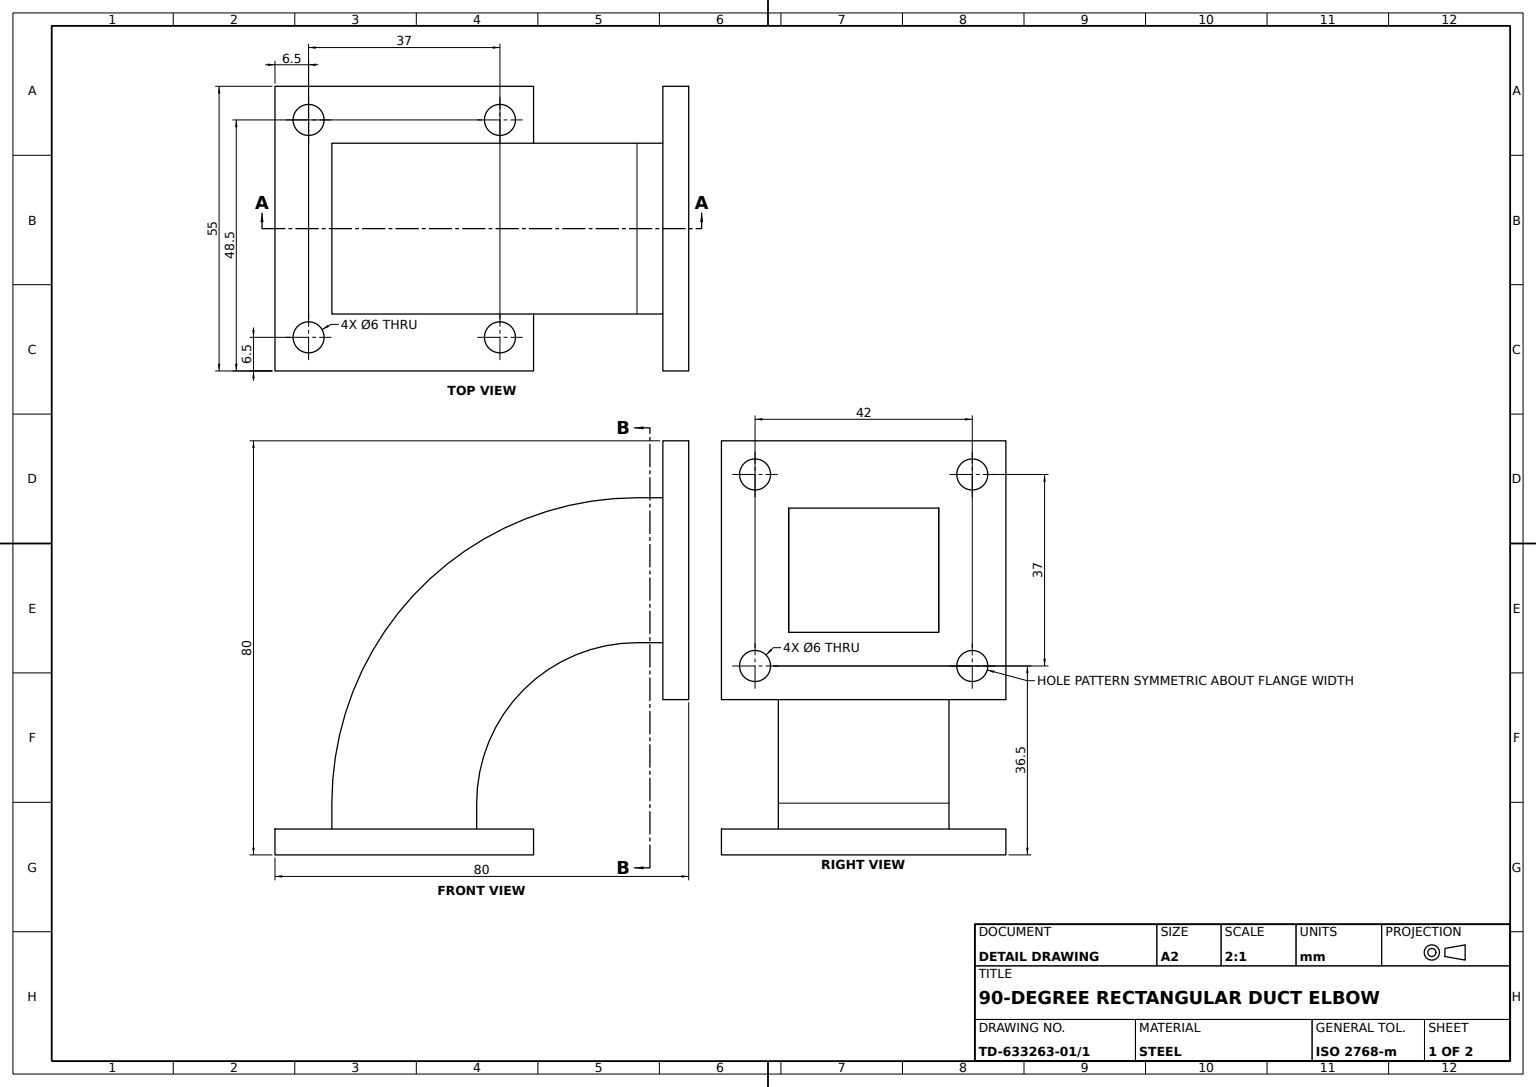
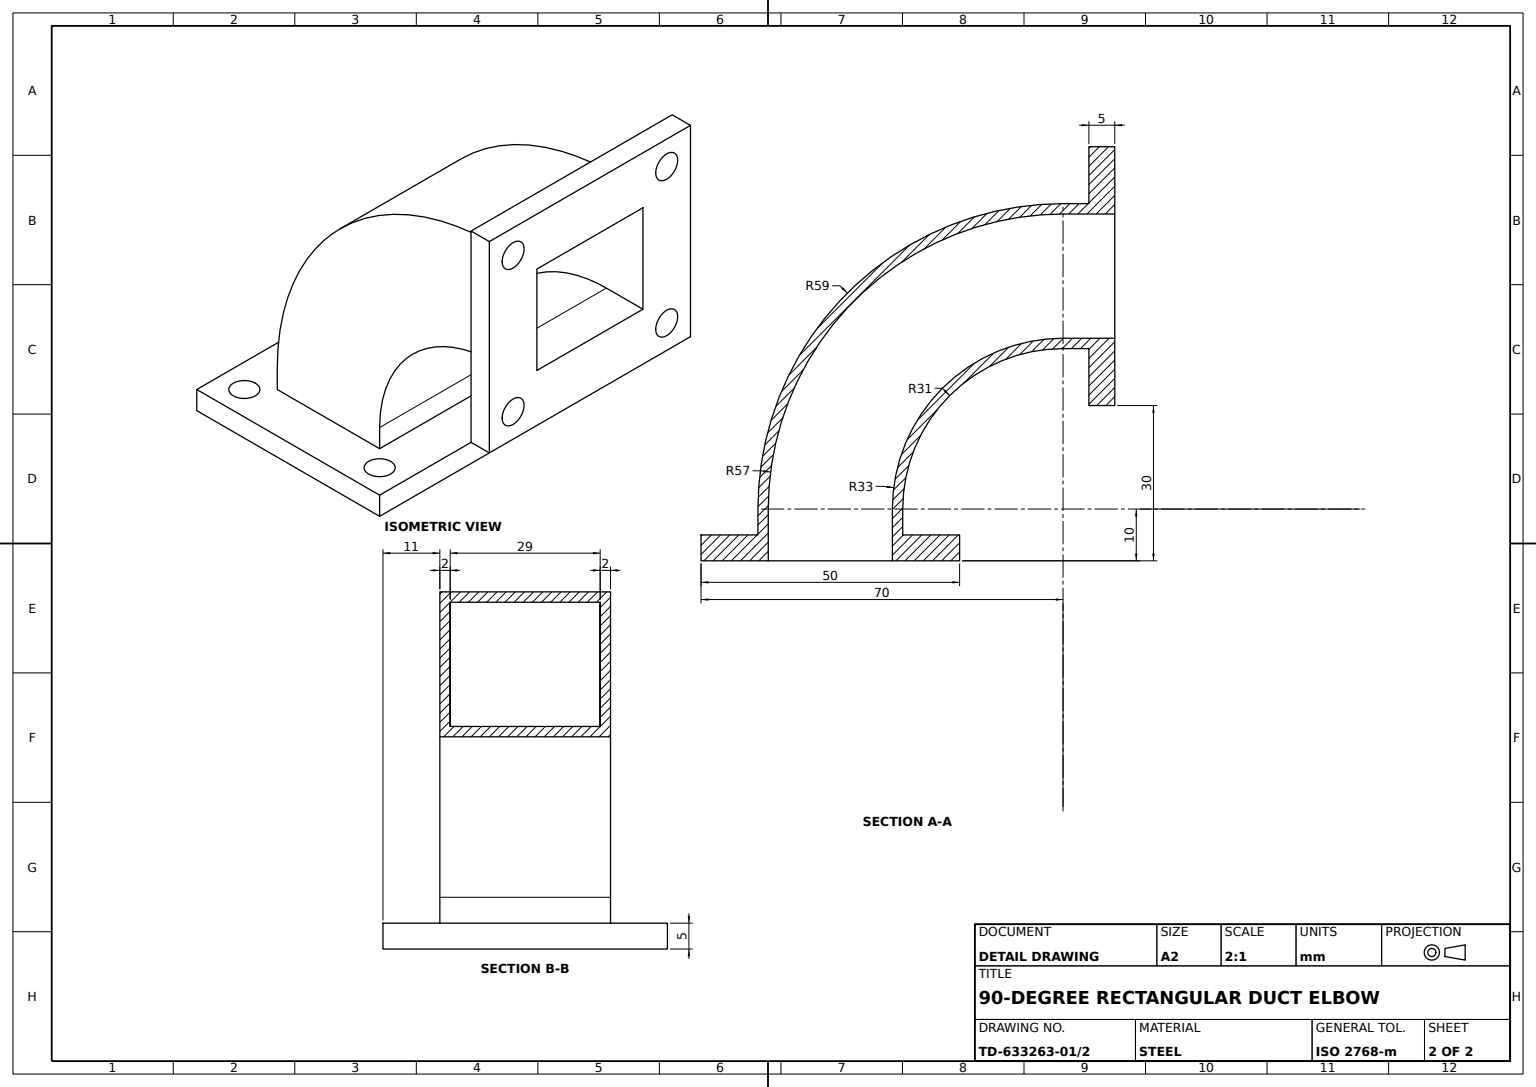
from build123d import *

# Parameters (mm, degrees)
INLET_FLANGE_SKETCH_W    = 55
INLET_FLANGE_SKETCH_H    = 50
INLET_FLANGE_SKETCH_R    = 3
INLET_FLANGE_SKETCH_W_2  = 29
INLET_FLANGE_SKETCH_H_2  = 24
INLET_FLANGE_5MM_DEPTH   = 5
OUTLET_FLANGE_SKETCH_W   = 50
OUTLET_FLANGE_SKETCH_H   = 55
OUTLET_FLANGE_SKETCH_R   = 3
OUTLET_FLANGE_SKETCH_W_2 = 24
OUTLET_FLANGE_SKETCH_H_2 = 29
OUTLET_FLANGE_5MM_DEPTH  = 5
BEND_PROFILE_SKETCH_W    = 28
BEND_PROFILE_SKETCH_H    = 33
BEND_PROFILE_SKETCH_W_2  = 24
BEND_PROFILE_SKETCH_H_2  = 29


with BuildPart() as part:
    # Inlet Flange Sketch → Inlet Flange 5mm (new body)
    with BuildSketch(Plane(origin=(0, 0, 0), x_dir=(0, 0, -1), z_dir=(1, 0, 0))):
        Rectangle(INLET_FLANGE_SKETCH_W, INLET_FLANGE_SKETCH_H)
        with Locations((-21, 18.5)):
            Circle(INLET_FLANGE_SKETCH_R, mode=Mode.SUBTRACT)
        with Locations((21, 18.5)):
            Circle(INLET_FLANGE_SKETCH_R, mode=Mode.SUBTRACT)
        with Locations((21, -18.5)):
            Circle(INLET_FLANGE_SKETCH_R, mode=Mode.SUBTRACT)
        with Locations((-21, -18.5)):
            Circle(INLET_FLANGE_SKETCH_R, mode=Mode.SUBTRACT)
        Rectangle(INLET_FLANGE_SKETCH_W_2, INLET_FLANGE_SKETCH_H_2, mode=Mode.SUBTRACT)
    extrude(amount=INLET_FLANGE_5MM_DEPTH)



with BuildPart() as body_2:
    # Outlet Flange Sketch → Outlet Flange 5mm (new body)
    with BuildSketch(Plane(origin=(0, -50, 0), x_dir=(1, 0, 0), z_dir=(0, 1, 0))):
        with Locations((-50, 0)):
            Rectangle(OUTLET_FLANGE_SKETCH_W, OUTLET_FLANGE_SKETCH_H)
        with Locations(Location((-68.5, 21, 0), (0, 0, 270))):
            Circle(OUTLET_FLANGE_SKETCH_R, mode=Mode.SUBTRACT)
        with Locations(Location((-31.5, 21, 0), (0, 0, 270))):
            Circle(OUTLET_FLANGE_SKETCH_R, mode=Mode.SUBTRACT)
        with Locations(Location((-31.5, -21, 0), (0, 0, 270))):
            Circle(OUTLET_FLANGE_SKETCH_R, mode=Mode.SUBTRACT)
        with Locations(Location((-68.5, -21, 0), (0, 0, 270))):
            Circle(OUTLET_FLANGE_SKETCH_R, mode=Mode.SUBTRACT)
        with Locations((-50, 0)):
            Rectangle(OUTLET_FLANGE_SKETCH_W_2, OUTLET_FLANGE_SKETCH_H_2, mode=Mode.SUBTRACT)
    extrude(amount=-OUTLET_FLANGE_5MM_DEPTH)


with BuildPart() as part_1:
    add(part.part)

    add(body_2.part)  # Elbow Bend Wall 2mm merges body 2
    # Elbow Bend Wall 2mm: sweep along a path in Bend Path R45 Sketch
    with BuildLine(Plane.XY) as elbow_bend_wall_2mm_path:
        Line((-50, -50), (-50, -45))
        ThreePointArc((-50, -45), (-36.819805153, -13.180194847), (-5, 0))
        Line((-5, 0), (0, 0))
    # Bend Profile Sketch → Elbow Bend Wall 2mm (sweep)
    with BuildSketch(Plane(origin=(0, -50, 0), x_dir=(1, 0, 0), z_dir=(0, 1, 0))):
        with Locations((-50, 0)):
            Rectangle(BEND_PROFILE_SKETCH_W, BEND_PROFILE_SKETCH_H)
        with Locations((-50, 0)):
            Rectangle(BEND_PROFILE_SKETCH_W_2, BEND_PROFILE_SKETCH_H_2, mode=Mode.SUBTRACT)
    sweep(path=elbow_bend_wall_2mm_path.line)


solid = part_1.part
